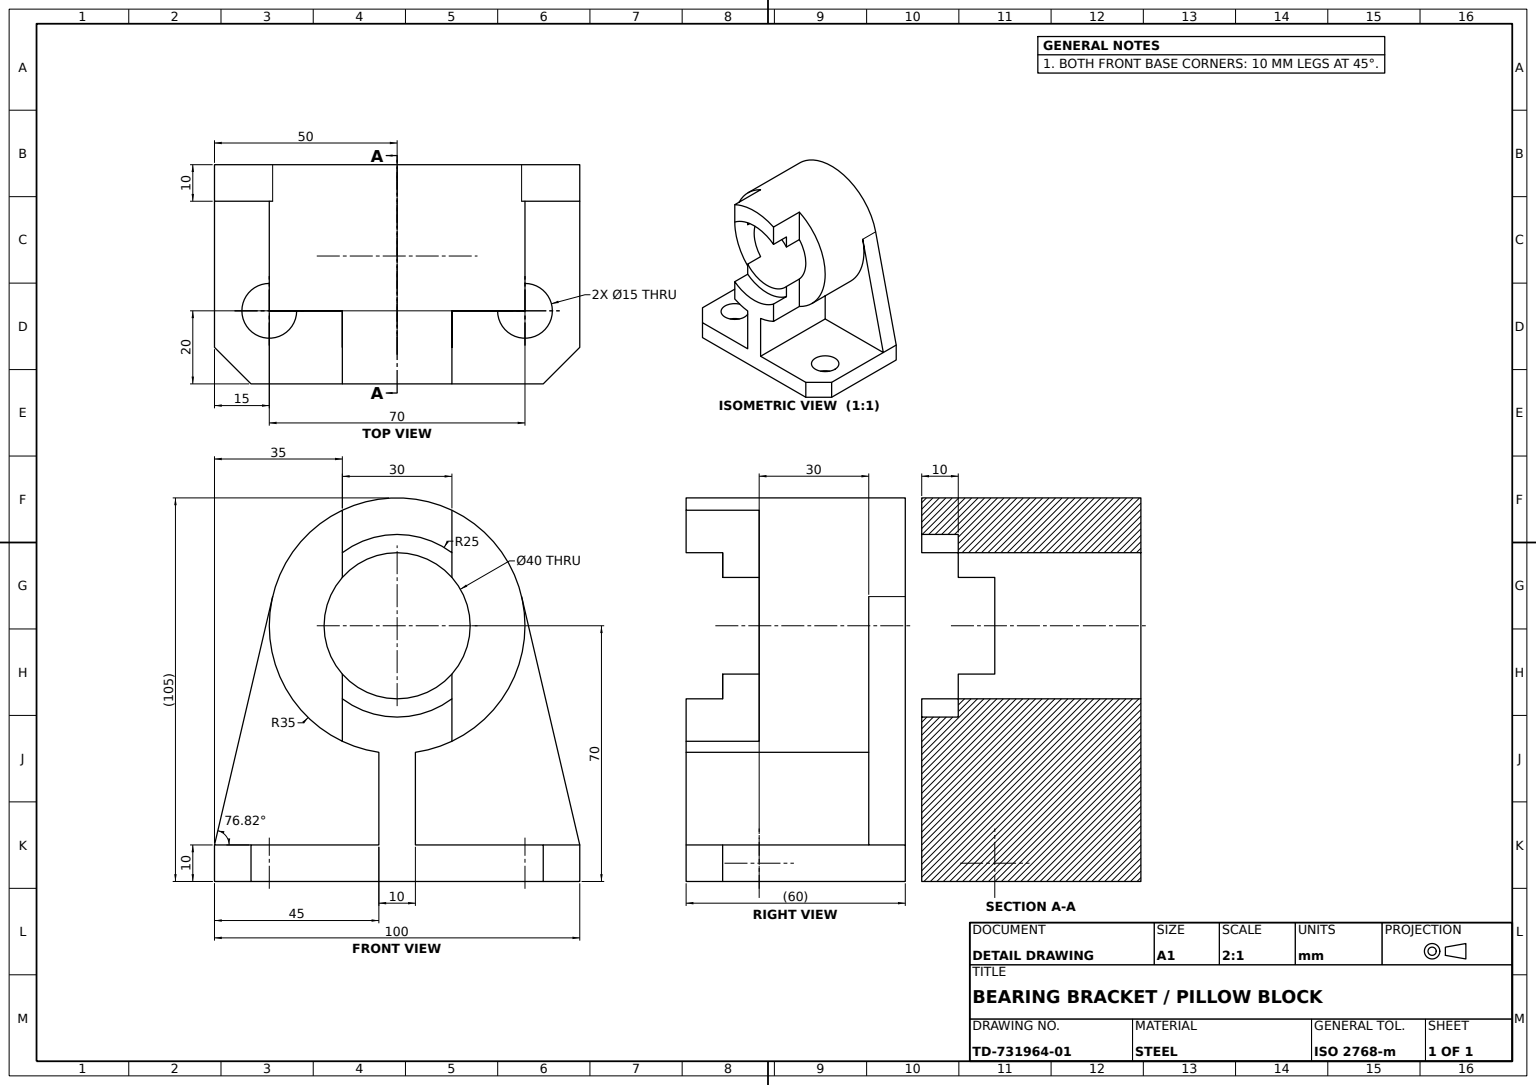
SolidWorks part; units mm, degrees
material "Plain Carbon Steel"
ref_plane "Front Plane" through (0, 0, 0) normal (0, 0, 1) x (1, 0, 0)
ref_plane "Top Plane" through (0, 0, 0) normal (0, 1, 0) x (1, 0, 0)
ref_plane "Right Plane" through (0, 0, 0) normal (1, 0, 0) x (0, 0, -1)
sketch "Back Plate Profile" plane through (0, 0, 0) normal (1, 0, 0) x (0, 0, -1)
  line L0 (-50, -70) -> (50, -70)
  line L1 (-50, -70) -> (-50, -60)
  line L3 (50, -60) -> (50, -70)
  line L4 (-50, -60) -> (-34.0778, 7.9815)
  line L5 (34.0778, 7.9815) -> (50, -60)
  arc A0 (34.0778, 7.9815) -> (-34.0778, 7.9815) centre (0, 0) ccw
  point P5 (0, -70)
  dimension "D1" = 35
  dimension "D2" = 100
  dimension "D3" = 10
  dimension "D4" = 70
extrude "Back Plate" add sketch "Back Plate Profile" along normal blind 10
sketch "Base Plate Profile" plane through (0, -70, 0) normal (0, -1, 0) x (1, 0, 0)
  line L0 (10, -50) -> (0, -50) construction
  line L1 (10, 50) -> (50, 50)
  line L2 (10, 50) -> (10, -50)
  line L3 (10, -50) -> (50, -50)
  line L4 (60, 40) -> (60, -40)
  line L5 (50, 50) -> (60, 40)
  line L6 (50, -50) -> (60, -40)
  point P1 (60, -50)
  point P3 (60, 50)
  dimension "D1" = 60
extrude "Base Plate" add sketch "Base Plate Profile" against normal blind 10
sketch "Housing Boss Profile" plane through (10, 0, 0) normal (1, 0, 0) x (0, 0, -1)
  line L0 (-50, -60) -> (50, -60) construction
  line L2 (-5, -34.641) -> (-5, -60)
  line L3 (-5, -60) -> (5, -60)
  line L4 (5, -34.641) -> (5, -60)
  arc A0 (5, -34.641) -> (-5, -34.641) centre (0, 0) ccw
  point P11 (0, -60)
  dimension "D2" = 35
  dimension "D1" = 10
extrude "Housing Boss" add sketch "Housing Boss Profile" along normal up to surface (50 mm away) up to face at (60, -65, 0)
sketch "Mounting Holes Sketch" plane through (0, -60, 0) normal (0, 1, 0) x (1, 0, 0)
  line L0 (10, 50) -> (50, 50) construction
  line L1 (60, -35) -> (60, 35) construction
  line L2 (0, 0) -> (66.4303, 0) construction
  circle A0 centre (40, 35) radius 7.5
  circle A1 centre (40, -35) radius 7.5
  dimension "D1" = 15
  dimension "D2" = 15
  dimension "D3" = 20
extrude "Mounting Holes" cut sketch "Mounting Holes Sketch" against normal up to next
sketch "Gland Bore Profile" plane through (0, 0, 0) normal (0, 0, 1) x (1, 0, 0)
  line L0 (0, 0) -> (60, 0)
  line L1 (60, 0) -> (60, 25)
  line L2 (60, 25) -> (50, 25)
  line L6 (40, 20) -> (0, 20)
  line L7 (0, 35) -> (0, 7.9815) construction
  line L8 (0, 20) -> (0, 0)
  line L9 (60, -34.641) -> (60, 35) construction
  line L10 (50, 25) -> (50, 20)
  line L11 (50, 20) -> (40, 20)
  dimension "D1" = 10
  dimension "D2" = 25
  dimension "D3" = 20
  dimension "D4" = 10
revolve "Gland Bore" cut sketch "Gland Bore Profile" angle 360 about L0
sketch "Housing Slot Profile" plane through (60, 0, 0) normal (1, 0, 0) x (0, 0, -1)
  line L0 (-34.0778, 7.9815) -> (-50, -60) construction
  line L1 (-15, 31.6228) -> (-43.3537, 31.6228)
  line L2 (-15, 31.6228) -> (-15, -31.6228)
  line L3 (-15, -31.6228) -> (-43.3537, -31.6228)
  line L4 (-43.3537, 31.6228) -> (-43.3537, -31.6228)
  line L5 (0, 0) -> (0, 44.9521) construction
  line L6 (15, -31.6228) -> (43.3537, -31.6228)
  line L7 (15, 31.6228) -> (15, -31.6228)
  line L8 (15, 31.6228) -> (43.3537, 31.6228)
  line L9 (43.3537, 31.6228) -> (43.3537, -31.6228)
  arc A0 (5, -34.641) -> (-5, -34.641) centre (0, 0) ccw construction
  arc A1 (-34.0778, 7.9815) -> (-5, -34.641) centre (0, 0) ccw construction
  arc A2 (5, -34.641) -> (34.0778, 7.9815) centre (0, 0) ccw construction
  dimension "D1" = 30
extrude "Housing Slot Cut" cut sketch "Housing Slot Profile" against normal blind 20
